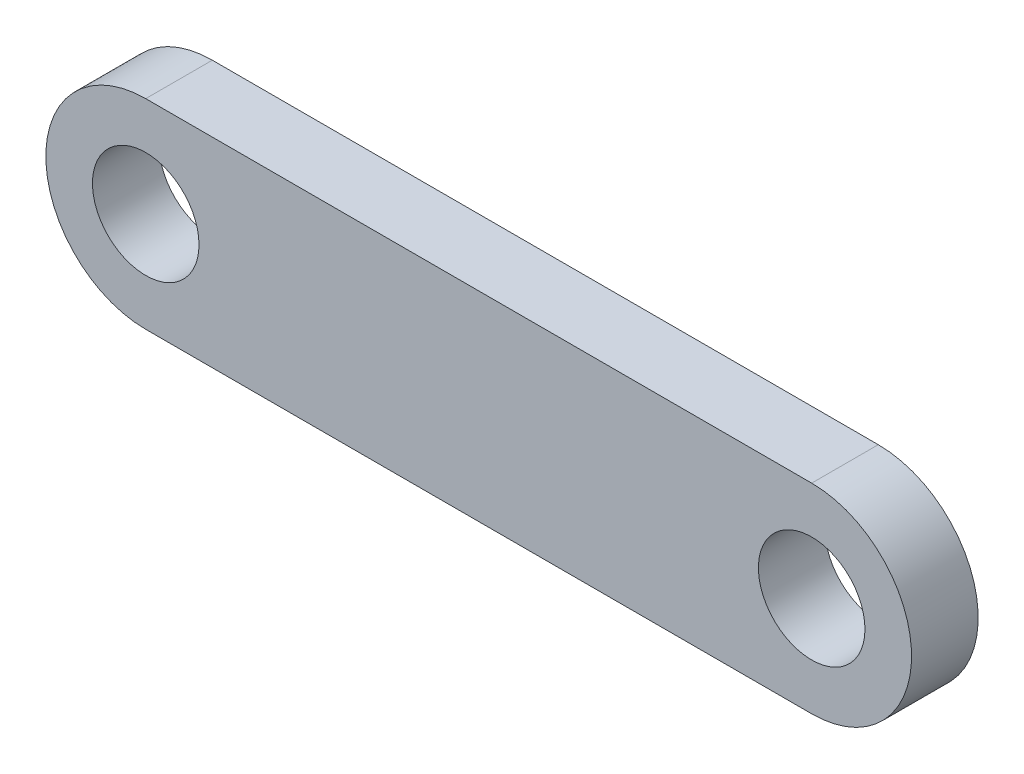
SolidWorks part; units mm, degrees
material "Plain Carbon Steel"
ref_plane "Front Plane" through (0, 0, 0) normal (0, 0, 1) x (1, 0, 0)
ref_plane "Top Plane" through (0, 0, 0) normal (0, 1, 0) x (1, 0, 0)
ref_plane "Right Plane" through (0, 0, 0) normal (1, 0, 0) x (0, 0, -1)
sketch "Link Plate Profile Sketch" plane through (0, 0, 0) normal (0, 0, 1) x (1, 0, 0)
  line L0 (25, 0) -> (-25, 0) construction
  line L1 (25, -7.5) -> (-25, -7.5)
  line L2 (25, 7.5) -> (-25, 7.5)
  arc A0 (25, -7.5) -> (25, 7.5) centre (25, 0) ccw
  arc A1 (-25, 7.5) -> (-25, -7.5) centre (-25, 0) ccw
  circle A2 centre (-25, 0) radius 4
  circle A3 centre (25, 0) radius 4
  point P2 (0, 0)
  dimension "D2" = 7.5
  dimension "D3" = 8
  dimension "D1" = 50
extrude "Link Plate 5mm with Holes 2xØ8" add sketch "Link Plate Profile Sketch" along normal mid plane 5
